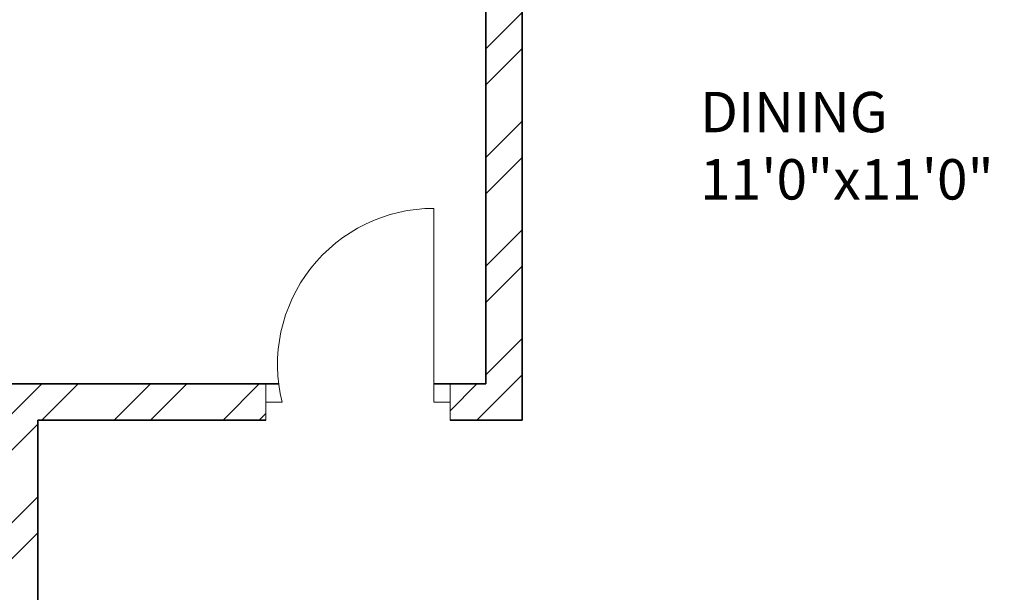
# Model space of a CAD drawing. Units: inches. Extents: x 1962 to 2771, y 1245 to 2660.
# Tile 4 of 114: x 2177 to 2299, y 1683 to 1753. Entities that reach past the tile are written whole.
import ezdxf

# ---------------------------------------------------------------- set-up
doc = ezdxf.new("R2010")
doc.units = ezdxf.units.IN
for name, color, linetype, lineweight in [('A-AREA-IDEN', 7, 'Continuous', 18), ('A-DOOR', 3, 'Continuous', 18), ('A-WALL', 7, 'Continuous', 35), ('A-WALL-PATT', 252, 'Continuous', 13)]:
    doc.layers.add(name, color=color, linetype=linetype, lineweight=lineweight)
doc.styles.get("Standard").update_dxf_attribs({"font": 'arial.ttf'})

msp = doc.modelspace()

# ---------------------------------------------------------------- hatches: boundary and pattern name
at = {"layer": 'A-WALL-PATT'}
h = msp.add_hatch(dxfattribs=at)
h.set_pattern_fill('ANSI32', color=256)
h.paths.add_polyline_path([(2090.8074, 2467.3437), (2141.6481, 2467.3437), (2141.6481, 2469.5937), (2141.6481, 2471.8437), (2086.3074, 2471.8437), (2086.3074, 2422.5333), (2090.8074, 2422.5333)])
h.paths.add_polyline_path([(2282.7664, 2471.8437), (2204.8982, 2471.8437), (2204.8982, 2467.3437), (2234.8074, 2467.3437), (2234.8074, 2311.3437), (2228.7492, 2311.3437), (2228.7492, 2306.8437), (2234.8074, 2306.8437), (2331.9227, 2306.8437), (2331.9227, 2309.0937), (2331.9227, 2311.3437), (2239.3074, 2311.3437), (2239.3074, 2467.3437), (2282.7664, 2467.3437), (2282.7664, 2469.5937)])
h.paths.add_polyline_path([(2471.4531, 2519.8437), (2552.011, 2519.8437), (2564.3996, 2519.8437), (2564.3996, 2511.1389), (2568.8996, 2511.1389), (2568.8996, 2524.3437), (2466.9531, 2524.3437), (2466.9531, 2471.8437), (2450.0749, 2471.8437), (2446.4672, 2471.8437), (2446.4672, 2467.3437), (2450.0749, 2467.3437), (2475.9988, 2467.3437), (2475.9988, 2469.5937), (2475.9988, 2471.8437), (2471.4531, 2471.8437)])
h.paths.add_polyline_path([(2575.2231, 2469.5937), (2575.2231, 2471.8437), (2568.8996, 2471.8437), (2568.8996, 2487.1389), (2564.3996, 2487.1389), (2564.3996, 2471.8437), (2556.511, 2471.8437), (2499.2904, 2471.8437), (2499.2904, 2467.3437), (2507.8074, 2467.3437), (2507.8074, 2311.3437), (2414.863, 2311.3437), (2414.863, 2306.8437), (2512.3074, 2306.8437), (2517.0114, 2306.8437), (2517.0114, 2309.0937), (2517.0114, 2311.3437), (2512.3074, 2311.3437), (2512.3074, 2467.3437), (2575.2231, 2467.3437)])
h.paths.add_polyline_path([(2660.8074, 2471.8437), (2600.9602, 2471.8437), (2600.9602, 2467.3437), (2656.3074, 2467.3437), (2656.3074, 2432.5704), (2660.8074, 2432.5704)])
h.paths.add_polyline_path([(2660.8074, 2372.5704), (2656.3074, 2372.5704), (2656.3074, 2311.3437), (2600.276, 2311.3437), (2600.276, 2309.0937), (2600.276, 2306.8437), (2656.3074, 2306.8437), (2656.3074, 2296.2593), (2660.8074, 2296.2593)])
h.paths.add_polyline_path([(2572.3074, 2306.8437), (2577.1385, 2306.8437), (2577.1385, 2311.3437), (2551.082, 2311.3437), (2551.082, 2306.8437), (2567.8074, 2306.8437), (2567.8074, 2258.8437), (2540.0574, 2258.8437), (2540.0574, 2256.5937), (2540.0574, 2254.3437), (2567.8074, 2254.3437), (2656.3074, 2254.3437), (2656.3074, 2236.9085), (2660.8074, 2236.9085), (2660.8074, 2272.2593), (2656.3074, 2272.2593), (2656.3074, 2258.8437), (2572.3074, 2258.8437)])
h.paths.add_polyline_path([(2512.3074, 2254.3437), (2518.8716, 2254.3437), (2518.8716, 2256.5937), (2518.8716, 2258.8437), (2507.8074, 2258.8437), (2507.8074, 2177.8437), (2567.8074, 2177.8437), (2567.8074, 2172.9628), (2572.3074, 2172.9628), (2572.3074, 2177.8437), (2656.3074, 2177.8437), (2656.3074, 2166.4846), (2660.8074, 2166.4846), (2660.8074, 2200.9085), (2656.3074, 2200.9085), (2656.3074, 2182.3437), (2512.3074, 2182.3437)])
h.paths.add_polyline_path([(2656.3074, 2129.8437), (2572.3074, 2129.8437), (2572.3074, 2150.3044), (2570.0574, 2150.3044), (2567.8074, 2150.3044), (2567.8074, 2129.8437), (2507.8074, 2129.8437), (2507.8074, 2116.3027), (2510.0574, 2116.3027), (2512.3074, 2116.3027), (2512.3074, 2125.3437), (2567.8074, 2125.3437), (2572.3074, 2125.3437), (2656.3074, 2125.3437)])
h.paths.add_polyline_path([(2090.8074, 2362.5333), (2086.3074, 2362.5333), (2086.3074, 2298.6242), (2090.8074, 2298.6242), (2090.8074, 2306.8437), (2174.8074, 2306.8437), (2174.8074, 2286.4178), (2179.3074, 2286.4178), (2179.3074, 2306.8437), (2192.8641, 2306.8437), (2192.8641, 2309.0937), (2192.8641, 2311.3437), (2090.8074, 2311.3437)])
h.paths.add_polyline_path([(2209.156, 2258.8437), (2179.3074, 2258.8437), (2179.3074, 2263.2236), (2177.0574, 2263.2236), (2174.8074, 2263.2236), (2174.8074, 2258.8437), (2090.8074, 2258.8437), (2090.8074, 2274.6242), (2086.3074, 2274.6242), (2086.3074, 2238.2967), (2088.5574, 2238.2967), (2090.8074, 2238.2967), (2090.8074, 2254.3437), (2209.156, 2254.3437)])
h.paths.add_polyline_path([(2090.8074, 2177.8437), (2234.8074, 2177.8437), (2234.8074, 2173.1428), (2239.3074, 2173.1428), (2239.3074, 2258.8437), (2230.8442, 2258.8437), (2230.8442, 2256.5937), (2230.8442, 2254.3437), (2234.8074, 2254.3437), (2234.8074, 2182.3437), (2090.8074, 2182.3437), (2090.8074, 2202.2967), (2086.3074, 2202.2967), (2086.3074, 2140.0389), (2090.8074, 2140.0389)])
h.paths.add_polyline_path([(2090.8074, 2080.0389), (2086.3074, 2080.0389), (2086.3074, 2033.8437), (2090.8074, 2033.8437)], flags=17)
h.paths.add_polyline_path([(2244.9405, 2033.8437), (2239.3074, 2033.8437), (2239.3074, 2142.0665), (2237.2592, 2142.0665), (2234.8074, 2142.0665), (2234.8074, 2033.8437), (2090.8074, 2033.8437), (2076.5204, 2033.8437), (2072.0204, 2033.8437), (2072.0204, 2000.4493), (2076.5204, 2000.4493), (2076.5204, 2029.3437), (2090.8074, 2029.3437), (2244.9405, 2029.3437), (2244.9405, 2031.5937)])
h.paths.add_polyline_path([(2234.8074, 1933.3437), (2076.5204, 1933.3437), (2076.5204, 1952.4493), (2074.2704, 1952.4493), (2072.0204, 1952.4493), (2072.0204, 1933.3437), (2072.0204, 1928.8437), (2234.8074, 1928.8437)])
h.paths.add_polyline_path([(2090.8074, 1928.8437), (2086.3074, 1928.8437), (2086.3074, 1906.5013), (2090.8074, 1906.5013)])
h.paths.add_polyline_path([(2090.8074, 1846.5013), (2086.3074, 1846.5013), (2086.3074, 1769.9917), (2088.5574, 1769.9917), (2090.8074, 1769.9917), (2090.8074, 1780.3437), (2234.8074, 1780.3437), (2234.8074, 1708.3437), (2230.3764, 1708.3437), (2230.3764, 1703.8437), (2239.3074, 1703.8437), (2239.3074, 1792.6669), (2237.0574, 1792.6669), (2234.8074, 1792.6669), (2234.8074, 1784.8437), (2090.8074, 1784.8437)])
h.paths.add_polyline_path([(2239.3074, 1928.8437), (2244.9405, 1928.8437), (2244.9405, 1931.0937), (2244.9405, 1933.3437), (2234.8074, 1933.3437), (2234.8074, 1928.8437), (2234.8074, 1825.5949), (2239.3074, 1825.5949)])
h.paths.add_polyline_path([(2148.0425, 1649.0937), (2148.0425, 1651.3437), (2090.8074, 1651.3437), (2090.8074, 1646.8437), (2148.0425, 1646.8437)], flags=0)
h.paths.add_polyline_path([(2207.5601, 1708.3437), (2090.8074, 1708.3437), (2090.8074, 1703.8437), (2174.8074, 1703.8437), (2174.8074, 1651.3437), (2170.4457, 1651.3437), (2170.4457, 1646.8437), (2195.9924, 1646.8437), (2195.9924, 1649.0937), (2195.9924, 1651.3437), (2179.3074, 1651.3437), (2179.3074, 1703.8437), (2207.5601, 1703.8437), (2207.5601, 1706.0937)])
h.paths.add_polyline_path([(2090.8074, 1733.9917), (2086.3074, 1733.9917), (2086.3074, 1696.1032), (2088.5574, 1696.1032), (2090.8074, 1696.1032)])
h.paths.add_polyline_path([(2090.8074, 1672.1032), (2086.3074, 1672.1032), (2086.3074, 1600.3335), (2090.8074, 1600.3335)])
h.paths.add_polyline_path([(2090.8074, 1540.3335), (2086.3074, 1540.3335), (2086.3074, 1486.3437), (2139.6766, 1486.3437), (2139.6766, 1490.8437), (2090.8074, 1490.8437)])
h.paths.add_polyline_path([(2302.3876, 1490.8437), (2239.3074, 1490.8437), (2239.3074, 1646.8437), (2335.9994, 1646.8437), (2335.9994, 1651.3437), (2229.884, 1651.3437), (2229.884, 1646.8437), (2234.8074, 1646.8437), (2234.8074, 1490.8437), (2202.7103, 1490.8437), (2202.7103, 1488.5937), (2202.7103, 1486.3437), (2275.0699, 1486.3437), (2275.0699, 1475.772), (2279.5699, 1475.772), (2279.5699, 1486.3437), (2302.3876, 1486.3437)])
h.paths.add_polyline_path([(2279.5699, 1451.772), (2275.0699, 1451.772), (2275.0699, 1438.3437), (2174.8074, 1438.3437), (2174.8074, 1486.3437), (2179.7922, 1486.3437), (2179.7922, 1490.8437), (2163.3585, 1490.8437), (2163.3585, 1488.5937), (2163.3585, 1486.3437), (2170.3074, 1486.3437), (2170.3074, 1433.8437), (2279.5699, 1433.8437)])
h.paths.add_polyline_path([(2427.2363, 1490.8437), (2375.8074, 1490.8437), (2375.8074, 1646.8437), (2381.6401, 1646.8437), (2381.6401, 1651.3437), (2365.887, 1651.3437), (2365.887, 1649.0937), (2365.887, 1646.8437), (2371.3074, 1646.8437), (2371.3074, 1490.8437), (2327.5627, 1490.8437), (2327.5627, 1488.5937), (2327.5627, 1486.3437), (2371.3074, 1486.3437), (2371.3074, 1433.8437), (2375.8074, 1433.8437), (2375.8074, 1486.3437), (2427.2363, 1486.3437)])
h.paths.add_polyline_path([(2512.3074, 1646.8437), (2519.4351, 1646.8437), (2519.4351, 1649.0937), (2519.4351, 1651.3437), (2507.8074, 1651.3437), (2416.0063, 1651.3437), (2416.0063, 1649.0937), (2416.0063, 1646.8437), (2507.8074, 1646.8437), (2507.8074, 1490.8437), (2497.0532, 1490.8437), (2497.0532, 1488.5937), (2497.0532, 1486.3437), (2574.9344, 1486.3437), (2574.9344, 1476.0181), (2579.4344, 1476.0181), (2579.4344, 1486.3437), (2584.4872, 1486.3437), (2584.3074, 1490.8437), (2512.3074, 1490.8437)])
h.paths.add_polyline_path([(2470.5091, 1486.3437), (2473.9767, 1486.3437), (2473.9767, 1490.8437), (2449.6605, 1490.8437), (2449.6605, 1488.5937), (2449.6605, 1486.3437), (2466.0091, 1486.3437), (2466.0091, 1433.8437), (2470.5091, 1433.8437), (2579.4344, 1433.8437), (2579.4344, 1452.0181), (2574.9344, 1452.0181), (2574.9344, 1438.3437), (2554.5091, 1438.3437), (2470.5091, 1438.3437)])
h.paths.add_polyline_path([(2656.3074, 1490.8437), (2611.86, 1490.8437), (2611.86, 1486.3437), (2656.3074, 1486.3437)])
h.paths.add_polyline_path([(2660.8074, 1532.7007), (2658.5574, 1532.7007), (2656.3074, 1532.7007), (2656.3074, 1486.3437), (2660.8074, 1486.3437)])
h.paths.add_polyline_path([(2660.8074, 1664.9663), (2656.3074, 1664.9663), (2656.3074, 1651.3437), (2602.2313, 1651.3437), (2602.2313, 1646.8437), (2656.3074, 1646.8437), (2656.3074, 1592.7007), (2660.8074, 1592.7007)])
h.paths.add_polyline_path([(2660.8074, 1724.5221), (2656.3074, 1724.5221), (2656.3074, 1703.8437), (2542.4725, 1703.8437), (2542.4725, 1699.3437), (2567.8074, 1699.3437), (2567.8074, 1651.3437), (2552.7766, 1651.3437), (2552.7766, 1649.0937), (2552.7766, 1646.8437), (2577.2878, 1646.8437), (2577.2878, 1649.0937), (2577.2878, 1651.3437), (2572.3074, 1651.3437), (2572.3074, 1699.3437), (2656.3074, 1699.3437), (2656.3074, 1688.9663), (2660.8074, 1688.9663)])
h.paths.add_polyline_path([(2660.8074, 1880.6524), (2656.3074, 1880.6524), (2656.3074, 1832.8437), (2512.3074, 1832.8437), (2512.3074, 1837.8959), (2507.8074, 1837.8959), (2507.8074, 1828.3437), (2567.8074, 1828.3437), (2567.8074, 1804.3437), (2572.3074, 1804.3437), (2572.3074, 1828.3437), (2656.3074, 1828.3437), (2656.3074, 1818.6778), (2660.8074, 1818.6778)])
h.paths.add_polyline_path([(2660.8074, 1794.6778), (2656.3074, 1794.6778), (2656.3074, 1780.3437), (2572.3074, 1780.3437), (2572.3074, 1783.0303), (2570.0574, 1783.0303), (2567.8074, 1783.0303), (2567.8074, 1780.3437), (2507.8074, 1780.3437), (2507.8074, 1699.3437), (2517.8858, 1699.3437), (2517.8858, 1701.5937), (2517.8858, 1703.8437), (2512.3074, 1703.8437), (2512.3074, 1775.8437), (2656.3074, 1775.8437), (2656.3074, 1760.5221), (2660.8074, 1760.5221)])
h.paths.add_polyline_path([(2660.8074, 1981.3437), (2660.8074, 2020.2808), (2658.5574, 2020.2808), (2656.3074, 2020.2808), (2656.3074, 1981.3437), (2512.3074, 1981.3437), (2512.3074, 2086.6996), (2507.8074, 2086.6996), (2507.8074, 1981.3437), (2375.8074, 1981.3437), (2375.8074, 1986.8505), (2373.5574, 1986.8505), (2371.3074, 1986.8505), (2371.3074, 1973.2607), (2375.8074, 1973.2607), (2375.8074, 1976.8437), (2507.8074, 1976.8437), (2507.8074, 1865.4281), (2510.0574, 1865.4281), (2512.3074, 1865.4281), (2512.3074, 1976.8437), (2660.8074, 1976.8437)])
h.paths.add_polyline_path([(2375.8074, 1940.297), (2373.5574, 1940.297), (2371.3074, 1940.297), (2371.3074, 1933.3437), (2278.4434, 1933.3437), (2278.4434, 1928.8437), (2371.3074, 1928.8437), (2371.3074, 1651.3437), (2375.8074, 1651.3437)])
h.paths.add_polyline_path([(2660.8074, 1976.8437), (2656.3074, 1976.8437), (2656.3074, 1940.6524), (2660.8074, 1940.6524)], flags=17)
h.paths.add_polyline_path([(2660.8074, 2142.4846), (2656.3074, 2142.4846), (2656.3074, 2080.2808), (2660.8074, 2080.2808)])
h.paths.add_polyline_path([(2381.4189, 2311.3437), (2375.8074, 2311.3437), (2375.8074, 2467.3437), (2424.7242, 2467.3437), (2424.7242, 2469.5937), (2424.7242, 2471.8437), (2375.8074, 2471.8437), (2375.8074, 2524.3437), (2371.3074, 2524.3437), (2371.3074, 2471.8437), (2307.2097, 2471.8437), (2307.2097, 2467.3437), (2371.3074, 2467.3437), (2371.3074, 2311.3437), (2366.8901, 2311.3437), (2366.8901, 2306.8437), (2371.3074, 2306.8437), (2371.3074, 2033.8437), (2279.6589, 2033.8437), (2279.6589, 2029.3437), (2371.3074, 2029.3437), (2371.3074, 2014.2598), (2375.8074, 2014.2598), (2375.8074, 2306.8437), (2381.4189, 2306.8437)])
h.paths.add_polyline_path([(2263.3074, 2524.3437), (2170.3074, 2524.3437), (2170.3074, 2519.8437), (2170.3074, 2471.8437), (2165.0312, 2471.8437), (2165.0312, 2467.3437), (2179.6721, 2467.3437), (2179.6721, 2469.5161), (2179.6721, 2471.8437), (2174.8074, 2471.8437), (2174.8074, 2519.8437), (2258.8074, 2519.8437), (2258.8074, 2511.6436), (2263.3074, 2511.6436)])
h.paths.add_polyline_path([(2245.0232, 1361.4123), (2492.9468, 1361.4123), (2492.9468, 1398.505), (2245.0232, 1398.505)], flags=9)
h.paths.add_polyline_path([(2388.1434, 2086.6936), (2425.0704, 2086.6936), (2425.0704, 2105.3509), (2388.1434, 2105.3509)], flags=9)
h.paths.add_polyline_path([(2404.922, 2242.6744), (2445.7337, 2242.6744), (2445.7337, 2261.3318), (2404.922, 2261.3318)], flags=9)
h.paths.add_polyline_path([(2269.4107, 2156.7935), (2306.3378, 2156.7935), (2306.3378, 2175.4508), (2269.4107, 2175.4508)], flags=9)
h.paths.add_polyline_path([(2269.3277, 2233.4343), (2306.2547, 2233.4343), (2306.2547, 2252.0917), (2269.3277, 2252.0917)], flags=9)
h.paths.add_polyline_path([(2431.6052, 2320.6922), (2470.4456, 2320.6922), (2470.4456, 2339.3495), (2431.6052, 2339.3495)], flags=25)
h.paths.add_polyline_path([(2249.6902, 2315.7608), (2288.5306, 2315.7608), (2288.5306, 2334.4182), (2249.6902, 2334.4182)], flags=25)
h.paths.add_polyline_path([(2096.9301, 2314.3181), (2135.7704, 2314.3181), (2135.7704, 2332.9755), (2096.9301, 2332.9755)], flags=25)
h.paths.add_polyline_path([(2134.3475, 2285.7089), (2161.4655, 2285.7089), (2161.4655, 2304.3662), (2134.3475, 2304.3662)], flags=9)
h.paths.add_polyline_path([(2126.5155, 2209.4076), (2159.9227, 2209.4076), (2159.9227, 2228.065), (2126.5155, 2228.065)], flags=25)
h.paths.add_polyline_path([(2110.5753, 2141.5299), (2149.4157, 2141.5299), (2149.4157, 2160.1872), (2110.5753, 2160.1872)], flags=25)
h.paths.add_polyline_path([(2249.8618, 1968.3317), (2286.3966, 1968.3317), (2286.3966, 1986.989), (2249.8618, 1986.989)], flags=9)
h.paths.add_polyline_path([(2395.9507, 1777.0051), (2436.7624, 1777.0051), (2436.7624, 1795.6625), (2395.9507, 1795.6625)], flags=9)
h.paths.add_polyline_path([(2398.5259, 1888.5651), (2435.0062, 1888.5651), (2435.0062, 1907.2224), (2398.5259, 1907.2224)], flags=25)
h.paths.add_polyline_path([(2259.3506, 1728.3559), (2296.2776, 1728.3559), (2296.2776, 1747.0132), (2259.3506, 1747.0132)], flags=9)
h.paths.add_polyline_path([(2271.3698, 1845.268), (2308.2968, 1845.268), (2308.2968, 1863.9253), (2271.3698, 1863.9253)], flags=9)
h.paths.add_polyline_path([(2120.9355, 1786.3027), (2159.7759, 1786.3027), (2159.7759, 1804.9601), (2120.9355, 1804.9601)], flags=25)
h.paths.add_polyline_path([(2121.3164, 1732.1043), (2154.7236, 1732.1043), (2154.7236, 1750.7616), (2121.3164, 1750.7616)], flags=25)
h.paths.add_polyline_path([(2118.3706, 1678.8997), (2147.5282, 1678.8997), (2147.5282, 1697.557), (2118.3706, 1697.557)], flags=25)
h.paths.add_polyline_path([(2385.9227, 1493.557), (2424.763, 1493.557), (2424.763, 1512.2143), (2385.9227, 1512.2143)], flags=25)
h.paths.add_polyline_path([(2248.7058, 1500.0256), (2287.5462, 1500.0256), (2287.5462, 1518.6829), (2248.7058, 1518.6829)], flags=25)
h.paths.add_polyline_path([(2104.1669, 1617.3771), (2143.0073, 1617.3771), (2143.0073, 1636.0344), (2104.1669, 1636.0344)], flags=9)
h.paths.add_polyline_path([(2096.0714, 1447.8824), (2137.3845, 1447.8824), (2137.3845, 1458.1859), (2096.0714, 1458.1859)], flags=9)
h.paths.add_polyline_path([(2180.6114, 1440.325), (2209.7689, 1440.325), (2209.7689, 1458.9823), (2180.6114, 1458.9823)], flags=25)
h.paths.add_polyline_path([(2316.1698, 1447.9637), (2357.4829, 1447.9637), (2357.4829, 1458.2673), (2316.1698, 1458.2673)], flags=9)
h.paths.add_polyline_path([(2397.6187, 1447.9637), (2438.9318, 1447.9637), (2438.9318, 1458.2673), (2397.6187, 1458.2673)], flags=9)
h.paths.add_polyline_path([(2473.0778, 1439.5953), (2502.2354, 1439.5953), (2502.2354, 1458.2527), (2473.0778, 1458.2527)], flags=25)
h.paths.add_polyline_path([(2589.7027, 1447.8819), (2631.0158, 1447.8819), (2631.0158, 1458.1855), (2589.7027, 1458.1855)], flags=9)
h.paths.add_polyline_path([(2522.4009, 1497.5285), (2561.2413, 1497.5285), (2561.2413, 1516.1859), (2522.4009, 1516.1859)], flags=25)
h.paths.add_polyline_path([(2579.6565, 1671.3482), (2608.8141, 1671.3482), (2608.8141, 1690.0056), (2579.6565, 1690.0056)], flags=25)
h.paths.add_polyline_path([(2544.7038, 1725.5064), (2578.1111, 1725.5064), (2578.1111, 1744.1637), (2544.7038, 1744.1637)], flags=25)
h.paths.add_polyline_path([(2578.1191, 1807.472), (2607.2766, 1807.472), (2607.2766, 1826.1293), (2578.1191, 1826.1293)], flags=25)
h.paths.add_polyline_path([(2595.0614, 1835.1839), (2633.9018, 1835.1839), (2633.9018, 1853.8413), (2595.0614, 1853.8413)], flags=25)
h.paths.add_polyline_path([(2567.0097, 2097.7035), (2605.8501, 2097.7035), (2605.8501, 2116.3609), (2567.0097, 2116.3609)], flags=9)
h.paths.add_polyline_path([(2586.644, 2134.6454), (2615.8015, 2134.6454), (2615.8015, 2153.3027), (2586.644, 2153.3027)], flags=9)
h.paths.add_polyline_path([(2544.6185, 2212.6783), (2578.0258, 2212.6783), (2578.0258, 2231.3356), (2544.6185, 2231.3356)], flags=25)
h.paths.add_polyline_path([(2577.0273, 2256.9023), (2606.1849, 2256.9023), (2606.1849, 2275.5597), (2577.0273, 2275.5597)], flags=24)
h.paths.add_polyline_path([(2605.2683, 2315.2821), (2644.1087, 2315.2821), (2644.1087, 2333.9395), (2605.2683, 2333.9395)], flags=25)
h.paths.add_polyline_path([(2583.1244, 2496.1815), (2624.4375, 2496.1815), (2624.4375, 2506.4851), (2583.1244, 2506.4851)], flags=9)
h.paths.add_polyline_path([(2474.761, 2497.0823), (2503.9185, 2497.0823), (2503.9185, 2515.7397), (2474.761, 2515.7397)], flags=25)
h.paths.add_polyline_path([(2387.5787, 2494.2563), (2428.902, 2494.2563), (2428.902, 2504.5598), (2387.5787, 2504.5598)], flags=9)
h.paths.add_polyline_path([(2300.1657, 2500.1564), (2341.4788, 2500.1564), (2341.4788, 2510.46), (2300.1657, 2510.46)], flags=25)
h.paths.add_polyline_path([(2176.8589, 2497.5843), (2206.0165, 2497.5843), (2206.0165, 2516.2416), (2176.8589, 2516.2416)], flags=25)
h.paths.add_polyline_path([(2097.4668, 2494.9762), (2138.7799, 2494.9762), (2138.7799, 2505.2798), (2097.4668, 2505.2798)], flags=9)

# ---------------------------------------------------------------- linework, layer by layer
at = {"layer": 'A-DOOR'}
for p, q in [((2228.3764, 1706.0937), (2228.3764, 1730.0937)), ((2207.5601, 1708.3437), (2207.5601, 1703.8437)), ((2230.3764, 1708.3437), (2230.3764, 1703.8437)), ((2207.5601, 1703.8437), (2207.5601, 1706.0937)), ((2207.5601, 1706.0937), (2209.5601, 1706.0937)), ((2230.3764, 1706.0937), (2228.3764, 1706.0937)), ((2230.3764, 1703.8437), (2230.3764, 1706.0937))]:
    msp.add_line(p, q, dxfattribs=at)
msp.add_arc((2228.3764, 1710.7176), 19.3761, 90, 193.806354, dxfattribs=at)
at = {"layer": 'A-WALL'}
for p, q in [((2239.3074, 1792.6669), (2239.3074, 1703.8437)), ((2234.8074, 1780.3437), (2234.8074, 1708.3437)), ((2090.8074, 1708.3437), (2209.1463, 1708.3437)), ((2228.3764, 1708.3437), (2234.8074, 1708.3437)), ((2179.3074, 1651.3437), (2179.3074, 1703.8437)), ((2179.3074, 1703.8437), (2207.5601, 1703.8437)), ((2230.3764, 1703.8437), (2239.3074, 1703.8437))]:
    msp.add_line(p, q, dxfattribs=at)

# ---------------------------------------------------------------- texts
at = {"layer": 'A-AREA-IDEN', "insert": (2261.3612, 1744.5251), "char_height": 5, "attachment_point": 1}
msp.add_mtext_dynamic_manual_height_columns('DINING\\P11\'0"x11\'0"', width=266.185845, gutter_width=12.5, heights=[0], dxfattribs=at)

doc.saveas('drawing.dxf')
